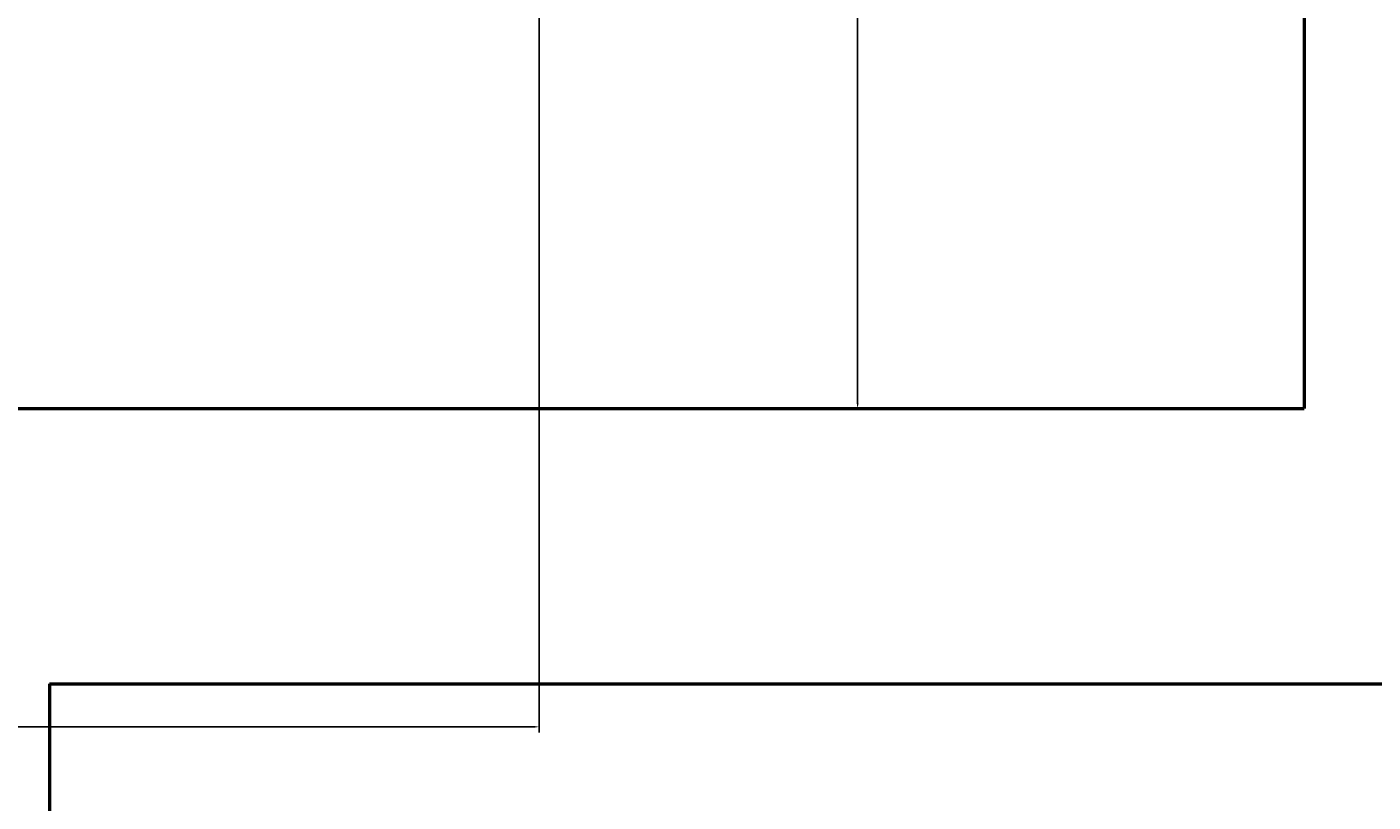
# Model space of a CAD drawing. Units: inches. Extents: x -173 to 545, y -746 to 104.
# Tile 26 of 32: x 219 to 263, y -94 to -69. Entities that reach past the tile are written whole.
import ezdxf

# ---------------------------------------------------------------- set-up
doc = ezdxf.new("R2010")
doc.units = ezdxf.units.IN
doc.header["$MEASUREMENT"] = 0
for name, color, linetype, lineweight in [('A-ANNO-DIMS', 2, 'Continuous', 18), ('A-FLOR-CASE', 9, 'Continuous', 25), ('A-WALL', 7, 'Continuous', 50)]:
    doc.layers.add(name, color=color, linetype=linetype, lineweight=lineweight)
doc.styles.get("Standard").update_dxf_attribs({"font": 'arial.ttf'})
doc.dimstyles.get("Standard").update_dxf_attribs({"dimtxt": 0.18, "dimasz": 0.18, "dimexe": 0.18, "dimexo": 0.0625, "dimgap": 0.09, "dimtad": 0, "dimtih": 1, "dimtoh": 1, "dimdec": 0, "dimzin": 0, "dimdsep": 46, "dimlunit": 3, "dimtxsty": 'Standard', "dimcen": 0.09, "dimadec": 0, "dimazin": 0, "dimtfac": 1, "dimtdec": 0, "dimtofl": 0, "dimtmove": 0, "dimatfit": 3, "dimfxl": 1, "dimtolj": 1, "dimtzin": 0, "dimarcsym": 0})

# ---------------------------------------------------------------- blocks, each defined once
blk = doc.blocks.new('COUNTER-L-RETURN')
blk.add_line((66, 0), (66, 69.362))
blk = doc.blocks.new('*D76')
at = {"layer": 'A-ANNO-DIMS', "color": 0, "lineweight": -2, "transparency": 16777216}
for p, q in [((235.864, -12), (246.386, -12)), ((246.206, -12.18), (246.206, -46.498)), ((246.206, -81.182), (246.206, -46.864)), ((235.864, -81.362), (246.386, -81.362))]:
    blk.add_line(p, q, dxfattribs=at)
at = {"layer": 'A-ANNO-DIMS', "color": 0, "transparency": 16777216}
for points in [[(246.176, -12.18), (246.236, -12.18), (246.206, -12)], [(246.176, -81.182), (246.236, -81.182), (246.206, -81.362)]]:
    blk.add_solid(points, dxfattribs=at)
at = {"layer": 'Defpoints', "color": 0, "transparency": 16777216}
for p in [(235.801, -12), (246.206, -12), (235.801, -81.362)]:
    blk.add_point(p, dxfattribs=at)
at = {"layer": 'A-ANNO-DIMS', "color": 0, "transparency": 16777216, "insert": (246.206, -46.681), "char_height": 0.18, "attachment_point": 5}
blk.add_mtext('\\A1;COUNTER 5\'-9 1/2" TYP.', dxfattribs=at)
blk = doc.blocks.new('*D77')
at = {"layer": 'A-ANNO-DIMS', "color": 0, "lineweight": -2, "transparency": 16777216}
for p, q in [((169.801, -81.424), (169.801, -91.946)), ((235.801, -81.424), (235.801, -91.946)), ((169.981, -91.766), (202.163, -91.766)), ((235.621, -91.766), (203.44, -91.766))]:
    blk.add_line(p, q, dxfattribs=at)
at = {"layer": 'A-ANNO-DIMS', "color": 0, "transparency": 16777216}
for points in [[(169.981, -91.736), (169.981, -91.796), (169.801, -91.766)], [(235.621, -91.736), (235.621, -91.796), (235.801, -91.766)]]:
    blk.add_solid(points, dxfattribs=at)
at = {"layer": 'Defpoints', "color": 0, "transparency": 16777216}
for p in [(169.801, -81.362), (235.801, -81.362), (235.801, -91.766)]:
    blk.add_point(p, dxfattribs=at)
at = {"layer": 'A-ANNO-DIMS', "color": 0, "transparency": 16777216, "insert": (202.801, -91.766), "char_height": 0.18, "attachment_point": 5}
blk.add_mtext('\\A1;5\'-6" TYP.', dxfattribs=at)

msp = doc.modelspace()

# ---------------------------------------------------------------- linework, layer by layer
at = {"layer": 'A-WALL'}
for p, q in [((260.801, 7.638), (260.801, -81.362)), ((210.801, -81.362), (260.801, -81.362)), ((219.801, -90.362), (260.801, -90.362)), ((219.801, -90.362), (219.801, -128.862)), ((260.801, -90.362), (265.301, -90.362))]:
    msp.add_line(p, q, dxfattribs=at)

# ---------------------------------------------------------------- block references
at = {"layer": 'A-FLOR-CASE'}
msp.add_blockref('COUNTER-L-RETURN', (169.801, -81.362), dxfattribs=at)

# ---------------------------------------------------------------- dimensions: what is measured, and where the dimension line sits
at = {"layer": 'A-ANNO-DIMS'}
dim = msp.add_linear_dim(base=(246.206, -12), p1=(235.801, -81.362), p2=(235.801, -12), angle=90, text='COUNTER <> TYP.', dimstyle='Standard', override={"dimdec": 1, "dimlfac": 1, "dimrnd": 0, "dimzin": 1, "dimdsep": 46, "dimlunit": 4, "dimfrac": 2}, dxfattribs=at)
dim.commit()
dim.dimension.update_dxf_attribs({"geometry": '*D76', "text_midpoint": (246.206, -46.681)})
dim = msp.add_linear_dim(base=(235.801, -91.766), p1=(169.801, -81.362), p2=(235.801, -81.362), text='<> TYP.', dimstyle='Standard', override={"dimdec": 1, "dimlfac": 1, "dimrnd": 0, "dimzin": 1, "dimdsep": 46, "dimlunit": 4, "dimfrac": 2}, dxfattribs=at)
dim.commit()
dim.dimension.update_dxf_attribs({"geometry": '*D77', "text_midpoint": (202.801, -91.766)})

doc.saveas('drawing.dxf')
